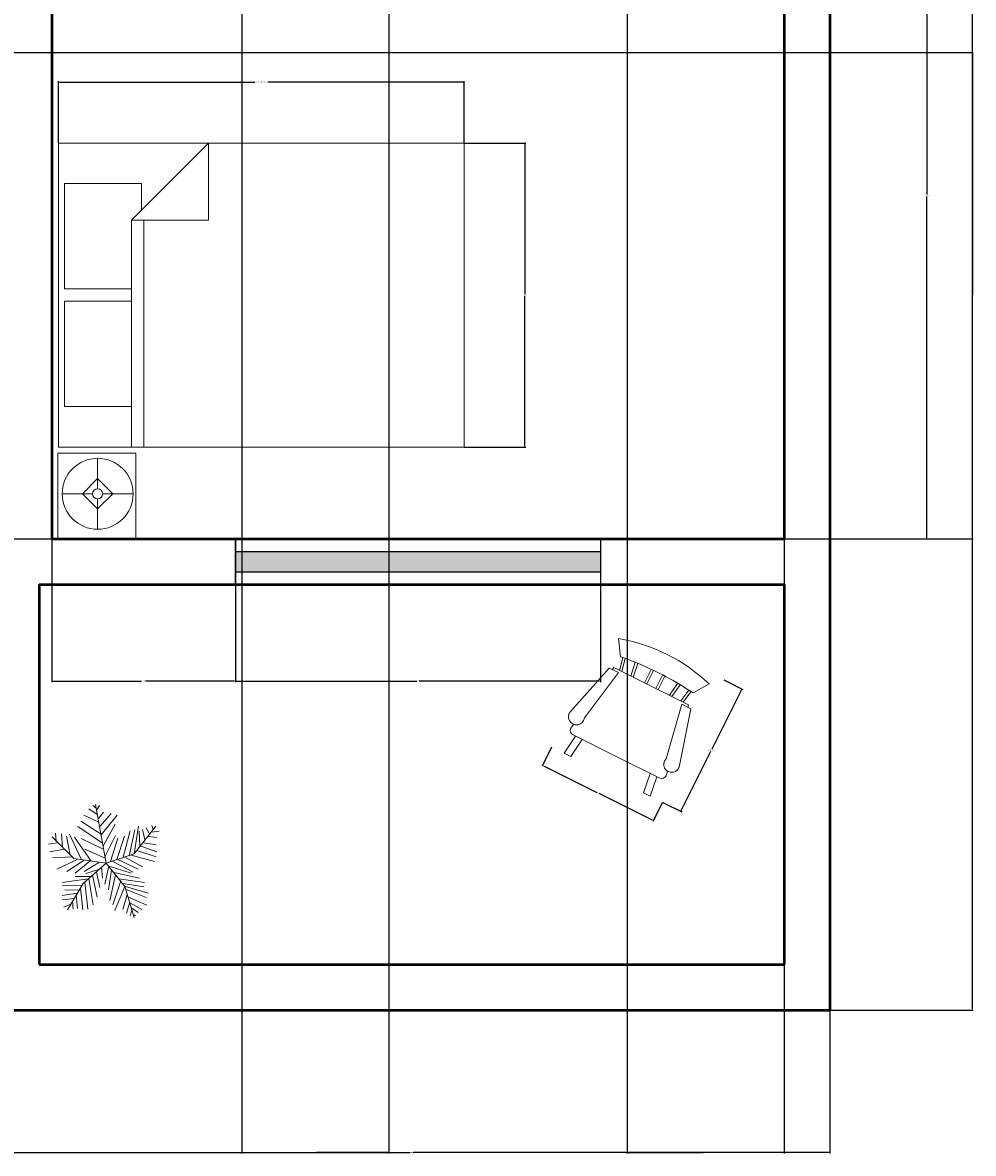
# Model space of a CAD drawing. Units: inches. Extents: x 1974 to 2406, y 1583 to 2170.
# Tile 2 of 6: x 2218 to 2406, y 1583 to 1806. Entities that reach past the tile are written whole.
import ezdxf

# ---------------------------------------------------------------- set-up
doc = ezdxf.new("R2010")
doc.units = ezdxf.units.IN
for name, color, linetype, lineweight in [('A-ANNO-DIMS', 2, 'Continuous', 18), ('A-FURN', 3, 'Continuous', 18), ('A-GLAZ', 4, 'Continuous', 25), ('A-GLAZ-PATT', 4, 'Continuous', 13), ('L-PLNT', 94, 'Continuous', 13), ('wall', 240, 'Continuous', 50)]:
    doc.layers.add(name, color=color, linetype=linetype, lineweight=lineweight)
doc.styles.get("Standard").update_dxf_attribs({"font": 'arial.ttf'})
doc.dimstyles.get("Standard").update_dxf_attribs({"dimtxt": 0.18, "dimasz": 0.18, "dimexe": 0.18, "dimexo": 0.0625, "dimgap": 0.09, "dimtad": 0, "dimtih": 1, "dimtoh": 1, "dimdec": 4, "dimzin": 0, "dimdsep": 46, "dimtxsty": 'Standard', "dimcen": 0.09, "dimadec": 0, "dimazin": 0, "dimtfac": 1, "dimtdec": 4, "dimtofl": 0, "dimtmove": 0, "dimatfit": 3, "dimfxl": 1, "dimtolj": 1, "dimtzin": 0, "dimarcsym": 0})

# ---------------------------------------------------------------- blocks, each defined once
blk = doc.blocks.new('Chair - Rocking')
for p, q in [((-8, -4.5), (-10, -1.5)), ((8, -4.5), (10, -1.5)), ((-6.5, -7), (-7.02225, -4.43)), ((-4.5, -7), (-4.96674, -4.19951)), ((-4, -7), (-4.40532, -4.16272)), ((-1.5, -4.05012), (-1.5, -7)), ((-1, -7), (-1, -4.05012)), ((1, -7), (1, -4.04655)), ((1.5, -4.05012), (1.5, -7)), ((4, -7), (4.40187, -4.18694)), ((4.5, -7), (4.96761, -4.19437)), ((6.5, -7), (7, -4.4057)), ((-7.5, -4.5), (-7, -7)), ((7.5, -4.5), (7, -7)), ((-9, -7.5), (-12, -18.49999)), ((-7, -7.5), (-9, -7.5)), ((-9, -18.49999), (-7, -7.5)), ((-8.23428, -6.99939), (-8.3093, -7.47958)), ((-8.23041, -7), (8.23915, -7)), ((7, -7.5), (9, -7.5)), ((9, -18.49999), (7, -7.5)), ((8.31071, -7.48854), (8.23449, -7.00073)), ((9, -7.5), (12, -18.49999)), ((-10.36644, -20.64523), (-10.5, -21.49999)), ((10.5, -21.49999), (10.3575, -20.58798)), ((-9, -22.49999), (-9.5, -26.49999)), ((0, -22.49999), (-9.5, -22.49999)), ((-8, -26.49999), (-7.5, -22.49999)), ((0, -22.49999), (9.5, -22.49999)), ((8, -26.49999), (7.5, -22.49999)), ((9, -22.49999), (9.5, -26.49999)), ((-9.5, -26.49999), (-8, -26.49999)), ((9.5, -26.49999), (8, -26.49999))]:
    blk.add_line(p, q)
for centre, radius, start, end in [((0, -34.08333), 34.08333, 72.93847, 107.0615), ((0, -68.25004), 64.25, 93.92211, 97.15267), ((0, -68.25004), 64.25, 82.84733, 93.92211), ((-10.5, -18.99999), 1.58114, 161.5651, 18.43495), ((10.5, -18.99999), 1.58114, 161.5651, 18.43495), ((-9.5, -21.49999), 1, 180, 270), ((9.5, -21.49999), 1, 270, 0)]:
    blk.add_arc(centre, radius, start, end)
blk = doc.blocks.new('Bed - Queen')
for p, q in [((0, -80.00003), (0, 0)), ((0, 0), (59.99999, 0)), ((59.99999, 0), (59.99999, -80.00003)), ((7.99999, -1.2), (28.79998, -1.2)), ((7.99999, -14.4), (7.99999, -1.2)), ((28.79998, -1.2), (28.79998, -14.4)), ((31.19999, -1.2), (51.99999, -1.2)), ((31.19999, -14.4), (31.19999, -1.2)), ((51.99999, -1.2), (51.99999, -16.4)), ((0, -14.4), (44.8, -14.4)), ((59.99999, -29.6), (44.8, -14.4)), ((44.8, -14.4), (44.8, -29.6)), ((44.8, -16.8), (0, -16.8)), ((51.99999, -16.4), (46.79936, -16.4)), ((44.8, -29.6), (59.99999, -29.6)), ((59.99999, -80.00003), (0, -80.00003))]:
    blk.add_line(p, q)
blk = doc.blocks.new('Lamp - Table')
for p, q in [((0, 7), (0, 1)), ((0, 3), (-3, 0)), ((3, 0), (0, 3)), ((-1, 0), (-7, 0)), ((-3, 0), (0, -3)), ((0, -3), (3, 0)), ((1, 0), (7, 0)), ((0, -1), (0, -7))]:
    blk.add_line(p, q)
for radius in [7, 1]:
    blk.add_circle((0, 0), radius)
blk = doc.blocks.new('Trees - Imperial')
for p, q in [((-10.186, 53.64), (-13.084, 55.962)), ((0, 0), (-10.5, 57)), ((-9.099, 51.782), (-6.563, 55.962)), ((-7.288, 39.707), (-21.778, 46.673)), ((-8.737, 47.138), (-17.069, 52.711)), ((-7.65, 43.423), (-2.578, 49.46)), ((-5.839, 35.992), (4.667, 48.067)), ((-5.114, 27.632), (10.463, 46.673)), ((-3.665, 19.273), (-27.574, 35.527)), ((-5.114, 28.097), (-24.676, 40.636)), ((-2.941, 16.486), (8.652, 37.85)), ((27, 9), (48, 36)), ((27.127, 9.056), (31.112, 35.992)), ((38.719, 34.134), (41.979, 28.561)), ((44.153, 36.456), (45.239, 32.741)), ((-31.5, 4.5), (-52.5, 25.5)), ((-48.585, 21.131), (-49.309, 29.026)), ((-43.513, 28.561), (-42.427, 15.558)), ((-38.442, 26.239), (-34.819, 7.663)), ((-35.544, 28.097), (-24.314, 3.947)), ((-14.533, 2.09), (-30.834, 25.31)), ((-24.314, 23.917), (-2.941, 13.7)), ((-1.129, 6.734), (9.014, 26.704)), ((3.942, 1.625), (11.187, 24.381)), ((10.101, 3.483), (17.708, 26.239)), ((16.259, 5.805), (23.142, 31.348)), ((22.055, 7.198), (27.489, 32.277)), ((31.836, 30.883), (32.561, 16.486)), ((35.096, 32.741), (37.27, 22.524)), ((40.53, 25.775), (48.862, 24.846)), ((43.791, 29.954), (51.036, 30.883)), ((-47.498, 19.737), (-55.83, 18.344)), ((-40.615, 13.7), (-55.105, 10.913)), ((-20.691, 13.7), (-1.129, 4.876)), ((29.662, 12.307), (48.137, 6.269)), ((33.285, 16.486), (48.862, 10.913)), ((36.183, 19.737), (48.137, 17.88)), ((-33.37, 6.269), (-52.207, 5.34)), ((-28.299, 3.483), (-47.86, -5.805)), ((-21.416, 3.018), (-38.079, -8.128)), ((0, 0), (-31.5, 4.5)), ((-15.982, 2.09), (-30.11, -9.521)), ((0, 0), (-22.5, -19.5)), ((-6.563, 1.161), (-21.416, -8.128)), ((0, 0), (27, 9)), ((0, 0), (18, -22.5)), ((6.478, 1.625), (26.04, -8.592)), ((11.187, 3.483), (30.749, -5.805)), ((18.07, 5.805), (35.096, -3.483)), ((24.229, 7.663), (46.688, 1.625)), ((-6.563, -5.805), (-19.967, -9.985)), ((-9.461, -8.592), (-6.201, -23.453)), ((-4.752, -3.483), (-3.665, -14.629)), ((2.493, -3.019), (-1.491, -20.202)), ((1.769, -2.555), (24.229, -9.521)), ((5.029, -6.27), (2.131, -25.775)), ((7.565, -9.056), (32.198, -14.629)), ((-17.431, -15.094), (-42.789, -18.809)), ((-24.314, -21.596), (-42.427, -22.06)), ((-22.5, -19.5), (-37.5, -45)), ((-15.257, -12.772), (-30.11, -12.772)), ((-20.691, -18.345), (-17.793, -44.352)), ((-17.069, -15.094), (-12.721, -40.172)), ((-13.446, -11.378), (-8.737, -32.741)), ((9.014, -11.378), (3.58, -35.992)), ((14.085, -16.951), (6.478, -40.172)), ((12.274, -15.094), (36.907, -18.809)), ((16.259, -19.738), (36.183, -22.989)), ((-28.299, -29.026), (-42.789, -31.348)), ((-26.849, -26.24), (-40.253, -25.775)), ((-29.023, -30.884), (-27.936, -43.887)), ((-25.038, -23.918), (-22.865, -45.281)), ((18.07, -22.524), (8.289, -45.745)), ((20.244, -30.419), (15.897, -44.816)), ((18, -22.5), (27, -52.5)), ((18.433, -22.524), (40.53, -29.026)), ((19.157, -25.311), (38.719, -33.206)), ((21.331, -32.741), (39.081, -40.636)), ((-30.834, -34.135), (-42.427, -35.528)), ((-34.457, -39.708), (-40.978, -42.494)), ((-32.646, -36.921), (-31.921, -44.352)), ((22.78, -37.85), (19.519, -48.532)), ((22.78, -38.314), (34.372, -44.816)), ((24.591, -43.423), (30.749, -47.603)), ((24.591, -45.745), (23.142, -50.854)), ((26.764, -49.925), (28.213, -50.854))]:
    blk.add_line(p, q)
blk = doc.blocks.new('TABLE-NIGHTSTAND')
blk.add_lwpolyline([(0, 15.39), (16.93, 15.39), (16.93, 0), (0, 0)], close=True)
blk = doc.blocks.new('*D28')
at = {"layer": 'A-ANNO-DIMS', "color": 0, "lineweight": -2, "transparency": 16777216}
for p, q in [((2225.49, 1782.16), (2225.49, 1794.28)), ((2225.67, 1794.1), (2264.19, 1794.1)), ((2305.31, 1794.1), (2266.79, 1794.1)), ((2305.49, 1782.16), (2305.49, 1794.28))]:
    blk.add_line(p, q, dxfattribs=at)
at = {"layer": 'A-ANNO-DIMS', "color": 0, "transparency": 16777216}
for points in [[(2225.67, 1794.13), (2225.67, 1794.07), (2225.49, 1794.1)], [(2305.31, 1794.13), (2305.31, 1794.07), (2305.49, 1794.1)]]:
    blk.add_solid(points, dxfattribs=at)
at = {"layer": 'Defpoints', "color": 0, "transparency": 16777216}
for p in [(2225.49, 1794.1), (2225.49, 1782.1), (2305.49, 1782.1)]:
    blk.add_point(p, dxfattribs=at)
at = {"layer": 'A-ANNO-DIMS', "color": 0, "transparency": 16777216, "insert": (2265.49, 1794.1), "char_height": 0.18, "attachment_point": 5}
blk.add_mtext('\\A1;QUEEN BED 80 TYP.', dxfattribs=at)
blk = doc.blocks.new('*D29')
at = {"layer": 'A-ANNO-DIMS', "color": 0, "lineweight": -2, "transparency": 16777216}
for p, q in [((2305.55, 1782.1), (2317.67, 1782.1)), ((2317.49, 1781.92), (2317.49, 1752.28)), ((2317.49, 1722.28), (2317.49, 1751.92)), ((2305.55, 1722.1), (2317.67, 1722.1))]:
    blk.add_line(p, q, dxfattribs=at)
at = {"layer": 'A-ANNO-DIMS', "color": 0, "transparency": 16777216}
for points in [[(2317.46, 1781.92), (2317.52, 1781.92), (2317.49, 1782.1)], [(2317.46, 1722.28), (2317.52, 1722.28), (2317.49, 1722.1)]]:
    blk.add_solid(points, dxfattribs=at)
at = {"layer": 'Defpoints', "color": 0, "transparency": 16777216}
for p in [(2305.49, 1782.1), (2317.49, 1782.1), (2305.49, 1722.1)]:
    blk.add_point(p, dxfattribs=at)
at = {"layer": 'A-ANNO-DIMS', "color": 0, "transparency": 16777216, "insert": (2317.49, 1752.1), "char_height": 0.18, "attachment_point": 5}
blk.add_mtext('\\A1;60 TYP.', dxfattribs=at)
blk = doc.blocks.new('*D40')
at = {"layer": 'A-ANNO-DIMS', "color": 0, "lineweight": -2, "transparency": 16777216}
for p, q in [((2356.77, 1676.13), (2360.5, 1674.26)), ((2360.26, 1674.18), (2354.4, 1662.45)), ((2348.35, 1650.35), (2354.21, 1662.08)), ((2344.71, 1651.97), (2348.43, 1650.11))]:
    blk.add_line(p, q, dxfattribs=at)
at = {"layer": 'A-ANNO-DIMS', "color": 0, "transparency": 16777216}
for points in [[(2360.23, 1674.2), (2360.28, 1674.17), (2360.34, 1674.34)], [(2348.33, 1650.36), (2348.38, 1650.34), (2348.27, 1650.19)]]:
    blk.add_solid(points, dxfattribs=at)
at = {"layer": 'Defpoints', "color": 0, "transparency": 16777216}
for p in [(2356.71, 1676.15), (2360.34, 1674.34), (2344.65, 1652)]:
    blk.add_point(p, dxfattribs=at)
at = {"layer": 'A-ANNO-DIMS', "color": 0, "transparency": 16777216, "insert": (2354.3, 1662.27), "char_height": 0.18, "attachment_point": 5}
blk.add_mtext('\\A1;ROCKER 27', dxfattribs=at)
blk = doc.blocks.new('*D41')
at = {"layer": 'A-ANNO-DIMS', "color": 0, "lineweight": -2, "transparency": 16777216}
for p, q in [((2322.76, 1662.86), (2320.9, 1659.13)), ((2321.14, 1659.21), (2331.69, 1653.94)), ((2342.68, 1648.45), (2332.13, 1653.72)), ((2344.62, 1651.94), (2342.76, 1648.21))]:
    blk.add_line(p, q, dxfattribs=at)
at = {"layer": 'A-ANNO-DIMS', "color": 0, "transparency": 16777216}
for points in [[(2321.15, 1659.24), (2321.13, 1659.18), (2320.98, 1659.29)], [(2342.69, 1648.48), (2342.67, 1648.43), (2342.84, 1648.37)]]:
    blk.add_solid(points, dxfattribs=at)
at = {"layer": 'Defpoints', "color": 0, "transparency": 16777216}
for p in [(2322.79, 1662.91), (2344.65, 1652), (2342.84, 1648.37)]:
    blk.add_point(p, dxfattribs=at)
at = {"layer": 'A-ANNO-DIMS', "color": 0, "transparency": 16777216, "insert": (2331.91, 1653.83), "char_height": 0.18, "attachment_point": 5}
blk.add_mtext('\\A1;24', dxfattribs=at)
blk = doc.blocks.new('*D49')
at = {"layer": 'A-ANNO-DIMS', "color": 0, "lineweight": -2, "transparency": 16777216}
for p, q in [((2377.72, 2141.99), (2405.96, 2141.99)), ((2405.78, 2141.81), (2405.78, 1876.67)), ((2405.78, 1611.17), (2405.78, 1876.31)), ((2377.72, 1610.99), (2405.96, 1610.99))]:
    blk.add_line(p, q, dxfattribs=at)
at = {"layer": 'A-ANNO-DIMS', "color": 0, "transparency": 16777216}
for points in [[(2405.75, 2141.81), (2405.81, 2141.81), (2405.78, 2141.99)], [(2405.75, 1611.17), (2405.81, 1611.17), (2405.78, 1610.99)]]:
    blk.add_solid(points, dxfattribs=at)
at = {"layer": 'Defpoints', "color": 0, "transparency": 16777216}
for p in [(2377.66, 2141.99), (2377.66, 1610.99), (2405.78, 1610.99)]:
    blk.add_point(p, dxfattribs=at)
at = {"layer": 'A-ANNO-DIMS', "color": 0, "transparency": 16777216, "insert": (2405.78, 1876.49), "char_height": 0.18, "attachment_point": 5}
blk.add_mtext('\\A1;531', dxfattribs=at)
blk = doc.blocks.new('*D60')
at = {"layer": 'A-ANNO-DIMS', "color": 0, "lineweight": -2, "transparency": 16777216}
for p, q in [((2368.72, 1839.49), (2396.96, 1839.49)), ((2396.78, 1839.31), (2396.78, 1771.92)), ((2396.78, 1704.17), (2396.78, 1771.56)), ((2368.72, 1703.99), (2396.96, 1703.99))]:
    blk.add_line(p, q, dxfattribs=at)
at = {"layer": 'A-ANNO-DIMS', "color": 0, "transparency": 16777216}
for points in [[(2396.75, 1839.31), (2396.81, 1839.31), (2396.78, 1839.49)], [(2396.75, 1704.17), (2396.81, 1704.17), (2396.78, 1703.99)]]:
    blk.add_solid(points, dxfattribs=at)
at = {"layer": 'Defpoints', "color": 0, "transparency": 16777216}
for p in [(2368.66, 1839.49), (2368.66, 1703.99), (2396.78, 1703.99)]:
    blk.add_point(p, dxfattribs=at)
at = {"layer": 'A-ANNO-DIMS', "color": 0, "transparency": 16777216, "insert": (2396.78, 1771.74), "char_height": 0.18, "attachment_point": 5}
blk.add_mtext('\\A1;135.5', dxfattribs=at)
blk = doc.blocks.new('*D62')
at = {"layer": 'A-ANNO-DIMS', "color": 0, "lineweight": -2, "transparency": 16777216}
for p, q in [((2212.66, 1610.93), (2212.66, 1582.69)), ((2377.66, 1610.93), (2377.66, 1582.69)), ((2212.84, 1582.87), (2294.88, 1582.87)), ((2377.48, 1582.87), (2295.44, 1582.87))]:
    blk.add_line(p, q, dxfattribs=at)
at = {"layer": 'A-ANNO-DIMS', "color": 0, "transparency": 16777216}
for points in [[(2212.84, 1582.9), (2212.84, 1582.84), (2212.66, 1582.87)], [(2377.48, 1582.9), (2377.48, 1582.84), (2377.66, 1582.87)]]:
    blk.add_solid(points, dxfattribs=at)
at = {"layer": 'Defpoints', "color": 0, "transparency": 16777216}
for p in [(2212.66, 1610.99), (2377.66, 1610.99), (2377.66, 1582.87)]:
    blk.add_point(p, dxfattribs=at)
at = {"layer": 'A-ANNO-DIMS', "color": 0, "transparency": 16777216, "insert": (2295.16, 1582.87), "char_height": 0.18, "attachment_point": 5}
blk.add_mtext('\\A1;165', dxfattribs=at)
blk = doc.blocks.new('*D63')
at = {"layer": 'A-ANNO-DIMS', "color": 0, "lineweight": -2, "transparency": 16777216}
for p, q in [((2260.41, 1703.93), (2260.41, 1675.69)), ((2332.41, 1703.93), (2332.41, 1675.69)), ((2260.59, 1675.87), (2296.19, 1675.87)), ((2332.23, 1675.87), (2296.63, 1675.87))]:
    blk.add_line(p, q, dxfattribs=at)
at = {"layer": 'A-ANNO-DIMS', "color": 0, "transparency": 16777216}
for points in [[(2260.59, 1675.9), (2260.59, 1675.84), (2260.41, 1675.87)], [(2332.23, 1675.9), (2332.23, 1675.84), (2332.41, 1675.87)]]:
    blk.add_solid(points, dxfattribs=at)
at = {"layer": 'Defpoints', "color": 0, "transparency": 16777216}
for p in [(2260.41, 1703.99), (2332.41, 1703.99), (2260.41, 1675.87)]:
    blk.add_point(p, dxfattribs=at)
at = {"layer": 'A-ANNO-DIMS', "color": 0, "transparency": 16777216, "insert": (2296.41, 1675.87), "char_height": 0.18, "attachment_point": 5}
blk.add_mtext('\\A1;72', dxfattribs=at)
blk = doc.blocks.new('*D64')
at = {"layer": 'A-ANNO-DIMS', "color": 0, "lineweight": -2, "transparency": 16777216}
for p, q in [((2224.16, 1703.93), (2224.16, 1675.69)), ((2260.41, 1703.93), (2260.41, 1675.69)), ((2224.34, 1675.87), (2241.89, 1675.87)), ((2260.23, 1675.87), (2242.68, 1675.87))]:
    blk.add_line(p, q, dxfattribs=at)
at = {"layer": 'A-ANNO-DIMS', "color": 0, "transparency": 16777216}
for points in [[(2224.34, 1675.9), (2224.34, 1675.84), (2224.16, 1675.87)], [(2260.23, 1675.9), (2260.23, 1675.84), (2260.41, 1675.87)]]:
    blk.add_solid(points, dxfattribs=at)
at = {"layer": 'Defpoints', "color": 0, "transparency": 16777216}
for p in [(2224.16, 1703.99), (2260.41, 1703.99), (2224.16, 1675.87)]:
    blk.add_point(p, dxfattribs=at)
at = {"layer": 'A-ANNO-DIMS', "color": 0, "transparency": 16777216, "insert": (2242.28, 1675.87), "char_height": 0.18, "attachment_point": 5}
blk.add_mtext('\\A1;36.25', dxfattribs=at)
blk = doc.blocks.new('*D76')
at = {"layer": 'A-ANNO-DIMS', "color": 0, "lineweight": -2, "transparency": 16777216}
for p, q in [((2261.66, 1839.43), (2261.66, 1582.69)), ((2290.66, 1839.43), (2290.66, 1582.69)), ((2261.84, 1582.87), (2275.94, 1582.87)), ((2290.48, 1582.87), (2276.38, 1582.87))]:
    blk.add_line(p, q, dxfattribs=at)
at = {"layer": 'A-ANNO-DIMS', "color": 0, "transparency": 16777216}
for points in [[(2261.84, 1582.9), (2261.84, 1582.84), (2261.66, 1582.87)], [(2290.48, 1582.9), (2290.48, 1582.84), (2290.66, 1582.87)]]:
    blk.add_solid(points, dxfattribs=at)
at = {"layer": 'Defpoints', "color": 0, "transparency": 16777216}
for p in [(2261.66, 1839.49), (2290.66, 1839.49), (2290.66, 1582.87)]:
    blk.add_point(p, dxfattribs=at)
at = {"layer": 'A-ANNO-DIMS', "color": 0, "transparency": 16777216, "insert": (2276.16, 1582.87), "char_height": 0.18, "attachment_point": 5}
blk.add_mtext('\\A1;29', dxfattribs=at)
blk = doc.blocks.new('*D79')
at = {"layer": 'A-ANNO-DIMS', "color": 0, "lineweight": -2, "transparency": 16777216}
for p, q in [((2368.66, 1905.93), (2368.66, 1582.69)), ((2337.66, 1901.93), (2337.66, 1582.69)), ((2337.84, 1582.87), (2352.7, 1582.87)), ((2368.48, 1582.87), (2353.62, 1582.87))]:
    blk.add_line(p, q, dxfattribs=at)
at = {"layer": 'A-ANNO-DIMS', "color": 0, "transparency": 16777216}
for points in [[(2337.84, 1582.9), (2337.84, 1582.84), (2337.66, 1582.87)], [(2368.48, 1582.9), (2368.48, 1582.84), (2368.66, 1582.87)]]:
    blk.add_solid(points, dxfattribs=at)
at = {"layer": 'Defpoints', "color": 0, "transparency": 16777216}
for p in [(2368.66, 1905.99), (2337.66, 1901.99), (2368.66, 1582.87)]:
    blk.add_point(p, dxfattribs=at)
at = {"layer": 'A-ANNO-DIMS', "color": 0, "transparency": 16777216, "insert": (2353.16, 1582.87), "char_height": 0.18, "attachment_point": 5}
blk.add_mtext('\\A1;30.994', dxfattribs=at)
blk = doc.blocks.new('*D86')
at = {"layer": 'A-ANNO-DIMS', "color": 0, "lineweight": -2, "transparency": 16777216}
for p, q in [((2215.22, 1799.99), (2405.96, 1799.99)), ((2405.78, 1799.81), (2405.78, 1752.17)), ((2405.78, 1704.17), (2405.78, 1751.81)), ((2215.22, 1703.99), (2405.96, 1703.99))]:
    blk.add_line(p, q, dxfattribs=at)
at = {"layer": 'A-ANNO-DIMS', "color": 0, "transparency": 16777216}
for points in [[(2405.75, 1799.81), (2405.81, 1799.81), (2405.78, 1799.99)], [(2405.75, 1704.17), (2405.81, 1704.17), (2405.78, 1703.99)]]:
    blk.add_solid(points, dxfattribs=at)
at = {"layer": 'Defpoints', "color": 0, "transparency": 16777216}
for p in [(2215.16, 1799.99), (2215.16, 1703.99), (2405.78, 1703.99)]:
    blk.add_point(p, dxfattribs=at)
at = {"layer": 'A-ANNO-DIMS', "color": 0, "transparency": 16777216, "insert": (2405.78, 1751.99), "char_height": 0.18, "attachment_point": 5}
blk.add_mtext('\\A1;96', dxfattribs=at)

msp = doc.modelspace()

# ---------------------------------------------------------------- hatches: boundary and pattern name
at = {"layer": 'A-GLAZ-PATT'}
h = msp.add_hatch(color=256, dxfattribs=at)
h.dxf.hatch_style = 1
h.paths.add_polyline_path([(2332.4081, 1701.4921), (2260.4081, 1701.4921), (2260.4081, 1697.4921), (2332.4081, 1697.4921)])

# ---------------------------------------------------------------- linework, layer by layer
at = {"layer": 'A-GLAZ'}
for p, q in [((2260.4081, 1701.4921), (2332.4081, 1701.4921)), ((2260.4081, 1697.4921), (2332.4081, 1697.4921))]:
    msp.add_line(p, q, dxfattribs=at)
msp.add_lwpolyline([(2260.4081, 1694.9921), (2260.4081, 1703.9921), (2332.4081, 1703.9921), (2332.4081, 1694.9921)], close=True, dxfattribs=at)
at = {"layer": 'wall'}
for p, q in [((2377.6581, 2141.9921), (2377.6581, 1610.9921)), ((2224.1581, 1839.4921), (2224.1581, 1703.9921)), ((2368.6581, 1839.4921), (2368.6581, 1703.9921)), ((2224.1581, 1703.9921), (2368.6581, 1703.9921)), ((2221.6581, 1694.9921), (2221.6581, 1619.9921)), ((2221.6581, 1694.9921), (2368.6581, 1694.9921)), ((2368.6581, 1694.9921), (2368.6581, 1619.9921)), ((2221.6581, 1619.9921), (2368.6581, 1619.9921)), ((2212.6581, 1610.9921), (2377.6581, 1610.9921))]:
    msp.add_line(p, q, dxfattribs=at)

# ---------------------------------------------------------------- block references
at = {"layer": 'A-FURN'}
for name, p, rotation in [('Bed - Queen', (2225.4913, 1722.1007), 90), ('TABLE-NIGHTSTAND', (2240.7583, 1703.9924), 90.00000000000281), ('Lamp - Table', (2233.2098, 1712.8735), 90), ('Chair - Rocking', (2345.5591, 1681.1645), 333.4631441252515)]:
    msp.add_blockref(name, p, dxfattribs=dict(at, rotation=rotation))
at = {"layer": 'L-PLNT', "xscale": 0.2037952239118122, "yscale": 0.2037952239118122, "zscale": 0.2037952239118122}
msp.add_blockref('Trees - Imperial', (2234.9164, 1639.9635), dxfattribs=at)

# ---------------------------------------------------------------- dimensions: what is measured, and where the dimension line sits
at = {"layer": 'A-ANNO-DIMS'}
for base, p1, p2, angle, override, picture, middle in [((2405.7756, 1610.9921), (2377.6581, 2141.9921), (2377.6581, 1610.9921), 90, {"dimdec": 0, "dimlfac": 1, "dimrnd": 0, "dimzin": 0, "dimdsep": 46, "dimlunit": 2}, '*D49', (2405.7756, 1876.4921)), ((2396.7756, 1703.9921), (2368.6581, 1839.4921), (2368.6581, 1703.9921), 270, {"dimdec": 1, "dimlfac": 1, "dimrnd": 0, "dimzin": 0, "dimdsep": 46, "dimlunit": 2}, '*D60', (2396.7756, 1771.7421)), ((2405.7756, 1703.9921), (2215.1581, 1799.9921), (2215.1581, 1703.9921), 90, {"dimdec": 0, "dimlfac": 1, "dimrnd": 0, "dimzin": 0, "dimdsep": 46, "dimlunit": 2}, '*D86', (2405.7756, 1751.9921)), ((2224.1581, 1675.8746), (2260.4081, 1703.9921), (2224.1581, 1703.9921), 180, {"dimdec": 2, "dimlfac": 1, "dimrnd": 0, "dimzin": 0, "dimdsep": 46, "dimlunit": 2}, '*D64', (2242.2831, 1675.8746)), ((2260.4081, 1675.8746), (2332.4081, 1703.9921), (2260.4081, 1703.9921), 180, {"dimdec": 0, "dimlfac": 1, "dimrnd": 0, "dimzin": 0, "dimdsep": 46, "dimlunit": 2}, '*D63', (2296.4081, 1675.8746)), ((2342.8406, 1648.3745), (2322.7892, 1662.9148), (2344.65, 1651.9978), 333.463144, {"dimdec": 0, "dimlfac": 1, "dimrnd": 0, "dimzin": 0, "dimdsep": 46, "dimlunit": 2}, '*D41', (2331.9102, 1653.833))]:
    dim = msp.add_linear_dim(base=base, p1=p1, p2=p2, angle=angle, dimstyle='Standard', override=override, dxfattribs=at)
    dim.commit()
    dim.dimension.update_dxf_attribs({"geometry": picture, "text_midpoint": middle})
for base, p1, p2, override, picture, middle in [((2368.6581, 1582.8746), (2337.6638, 1901.9921), (2368.6581, 1905.9921), {"dimdec": 3, "dimlfac": 1, "dimrnd": 0, "dimzin": 0, "dimdsep": 46, "dimlunit": 2}, '*D79', (2353.1609, 1582.8746)), ((2290.6581, 1582.8746), (2261.6581, 1839.4921), (2290.6581, 1839.4921), {"dimdec": 0, "dimlfac": 1, "dimrnd": 0, "dimzin": 0, "dimdsep": 46, "dimlunit": 2}, '*D76', (2276.1581, 1582.8746)), ((2377.6581, 1582.8746), (2212.6581, 1610.9921), (2377.6581, 1610.9921), {"dimdec": 0, "dimlfac": 1, "dimrnd": 0, "dimzin": 0, "dimdsep": 46, "dimlunit": 2}, '*D62', (2295.1581, 1582.8746))]:
    dim = msp.add_linear_dim(base=base, p1=p1, p2=p2, dimstyle='Standard', override=override, dxfattribs=at)
    dim.commit()
    dim.dimension.update_dxf_attribs({"geometry": picture, "text_midpoint": middle})
for base, p1, p2, angle, text, picture, middle in [((2225.4913, 1794.1007), (2305.4913, 1782.1007), (2225.4913, 1782.1007), 180, 'QUEEN BED <> TYP.', '*D28', (2265.4913, 1794.1007)), ((2317.4913, 1782.1007), (2305.4913, 1722.1007), (2305.4913, 1782.1007), 90, '<> TYP.', '*D29', (2317.4913, 1752.1007)), ((2360.3362, 1674.3439), (2344.65, 1651.9978), (2356.7129, 1676.1533), 63.463144, 'ROCKER <>', '*D40', (2354.3048, 1662.2661))]:
    dim = msp.add_linear_dim(base=base, p1=p1, p2=p2, angle=angle, text=text, dimstyle='Standard', override={"dimdec": 0, "dimlfac": 1, "dimrnd": 0, "dimzin": 0, "dimdsep": 46, "dimlunit": 2}, dxfattribs=at)
    dim.commit()
    dim.dimension.update_dxf_attribs({"geometry": picture, "text_midpoint": middle})

doc.saveas('drawing.dxf')
